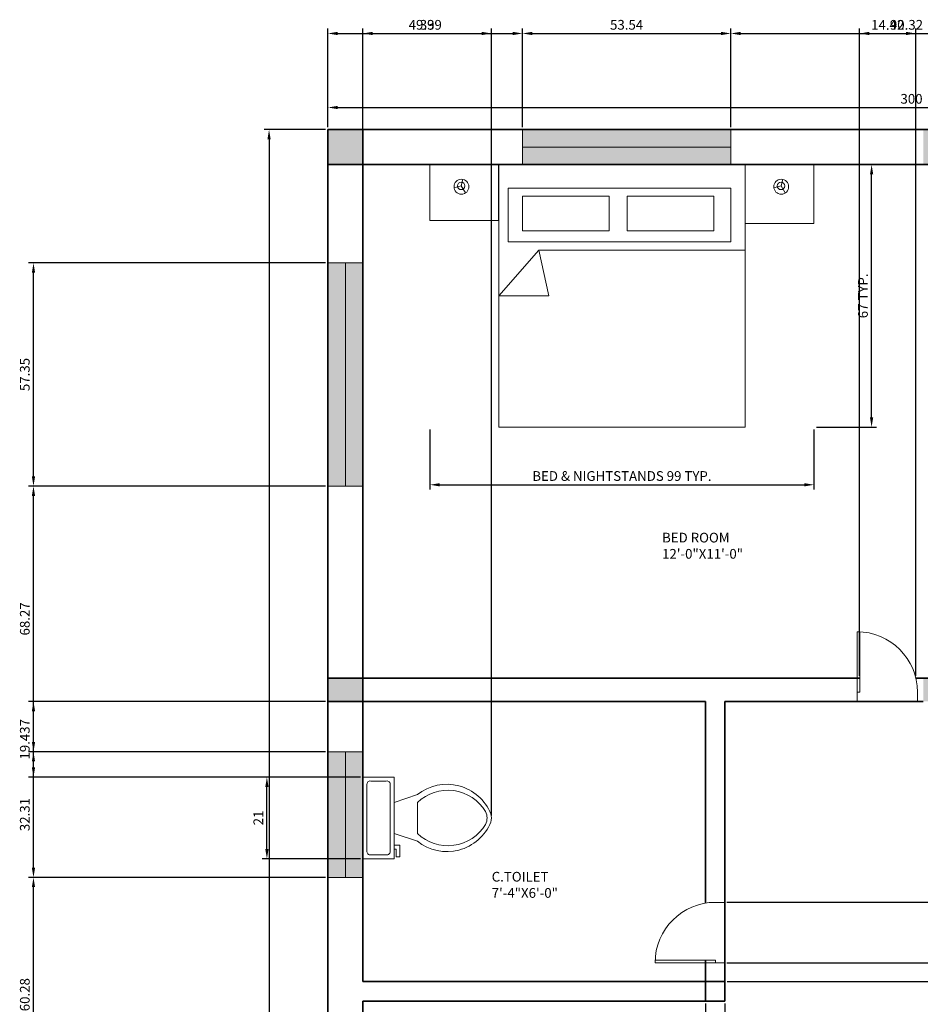
# Model space of a CAD drawing. Units: inches. Extents: x 33934 to 34340, y 20959 to 21493.
# Tile 3 of 4: x 33934 to 34166, y 21240 to 21493. Entities that reach past the tile are written whole.
import ezdxf

# ---------------------------------------------------------------- set-up
doc = ezdxf.new("R2010")
doc.units = ezdxf.units.IN
for name, color, linetype, lineweight in [('A-ANNO-DIMS', 2, 'Continuous', 18), ('A-AREA-IDEN', 7, 'Continuous', 18), ('A-DOOR', 3, 'Continuous', 18), ('A-FLOR-FIXT', 9, 'Continuous', 18), ('A-FURN', 8, 'Continuous', 18), ('A-GLAZ', 4, 'Continuous', 18), ('A-WALL', 7, 'Continuous', 35)]:
    doc.layers.add(name, color=color, linetype=linetype, lineweight=lineweight)
doc.layers.add('A-COLS-PATT', color=141, linetype='Continuous', lineweight=13, true_color=0xadddf7)
doc.layers.add('A-GLAZ-PATT', color=159, linetype='Continuous', lineweight=13, true_color=0x22346e)
doc.styles.get("Standard").update_dxf_attribs({"font": 'arial.ttf'})
doc.dimstyles.new('ISO-25', dxfattribs={"dimtxt": 2.5, "dimasz": 2.5, "dimexe": 1.25, "dimexo": 0.625, "dimtad": 1, "dimtxsty": 'Standard', "dimcen": 2.5, "dimadec": 0, "dimazin": 0, "dimtfac": 1, "dimtmove": 0, "dimatfit": 3, "dimfxl": 1, "dimarcsym": 0})

# ---------------------------------------------------------------- blocks, each defined once
blk = doc.blocks.new('*U3')
for p, q in [((9.5, -6), (9.5, -2)), ((-10, -8.5), (-8, -8.5)), ((-10, -9.5), (-10, -8.5)), ((-7, -9.5), (-10, -9.5)), ((-8, -8.5), (-8, -8)), ((-7, -8), (-7, -9.5)), ((-4, -8), (-6, -14)), ((4, -8), (6, -14)), ((4, -14), (-4, -14))]:
    blk.add_line(p, q)
blk.add_lwpolyline([(10.5, -8), (10.5, 0), (-10.5, 0), (-10.5, -8)], close=True)
for points in [[(-9.5, -2), (-9.5, -6)], [(8.5, -1), (-8.5, -1)], [(-8.5, -7), (8.5, -7)]]:
    blk.add_lwpolyline(points)
for centre, radius, start, end in [((-8.62, -1.88), 0.884, 81.8699, 188.1301), ((8.62, -1.88), 0.884, 351.8699, 98.1301), ((-8.62, -6.12), 0.884, 171.8699, 278.1301), ((8.62, -6.12), 0.884, 261.8699, 8.1301), ((3.52, -21.58), 12.17, 141.4691, 247.9714), ((4.2, -21.82), 11.33, 136.3677, 238.9468), ((-3.52, -21.58), 12.17, 292.0284, 38.5307), ((-4.2, -21.82), 11.33, 301.053, 43.6321), ((0, -27.88), 4, 245.7318, 294.2682), ((0, -29), 4, 254.8605, 285.1395)]:
    blk.add_arc(centre, radius, start, end)
blk = doc.blocks.new('*U5')
for p, q in [((0, 0), (0, -6)), ((40, 0), (40, -6))]:
    blk.add_line(p, q)
blk.add_lwpolyline([(0, 0), (0, 40), (1.75, 40), (1.75, 0)], close=True)
blk.add_arc((0, 0), 40, 0, 90)
blk = doc.blocks.new('*D6')
at = {"layer": 'A-ANNO-DIMS', "color": 0, "lineweight": -2, "transparency": 16777216}
for p, q in [((34013.69, 21465.74), (34013.69, 21472.03)), ((34313.69, 21465.74), (34313.69, 21472.03)), ((34016.19, 21470.78), (34311.19, 21470.78))]:
    blk.add_line(p, q, dxfattribs=at)
at = {"layer": 'A-ANNO-DIMS', "color": 0, "transparency": 16777216}
for points in [[(34016.19, 21471.2), (34016.19, 21470.37), (34013.69, 21470.78)], [(34311.19, 21471.2), (34311.19, 21470.37), (34313.69, 21470.78)]]:
    blk.add_solid(points, dxfattribs=at)
at = {"layer": 'Defpoints', "color": 0, "transparency": 16777216}
for p in [(34313.69, 21470.78), (34013.69, 21465.11), (34313.69, 21465.11)]:
    blk.add_point(p, dxfattribs=at)
at = {"layer": 'A-ANNO-DIMS', "color": 0, "transparency": 16777216, "insert": (34163.69, 21472.69), "char_height": 2.5, "attachment_point": 5}
blk.add_mtext('300', dxfattribs=at)
blk = doc.blocks.new('*D7')
at = {"layer": 'A-ANNO-DIMS', "color": 0, "lineweight": -2, "transparency": 16777216}
for p, q in [((34013.07, 21465.11), (33997.3, 21465.11)), ((33998.55, 21462.61), (33998.55, 20987.61)), ((34013.07, 20985.11), (33997.3, 20985.11))]:
    blk.add_line(p, q, dxfattribs=at)
at = {"layer": 'A-ANNO-DIMS', "color": 0, "transparency": 16777216}
for points in [[(33998.13, 21462.61), (33998.96, 21462.61), (33998.55, 21465.11)], [(33998.13, 20987.61), (33998.96, 20987.61), (33998.55, 20985.11)]]:
    blk.add_solid(points, dxfattribs=at)
at = {"layer": 'Defpoints', "color": 0, "transparency": 16777216}
for p in [(34013.69, 21465.11), (33998.55, 20985.11), (34013.69, 20985.11)]:
    blk.add_point(p, dxfattribs=at)
at = {"layer": 'A-ANNO-DIMS', "color": 0, "transparency": 16777216, "insert": (33996.64, 21225.11), "char_height": 2.5, "attachment_point": 5, "rotation": 90}
blk.add_mtext('480', dxfattribs=at)
blk = doc.blocks.new('BED-DOUBLE-WITH-NIGHTSTANDS')
for p, q in [((-9.63, -5.48), (-9.19, -3.82)), ((72.57, -5.48), (73, -3.82)), ((-9.63, -5.48), (-11.46, -5.95)), ((-9.63, -5.48), (-8.53, -7.28)), ((72.57, -5.48), (70.73, -5.95)), ((72.57, -5.48), (73.67, -7.28)), ((10.3, -21.96), (0, -33.74)), ((63.37, -21.96), (10.3, -21.96)), ((12.88, -33.74), (10.3, -21.96)), ((0, -33.74), (12.88, -33.74))]:
    blk.add_line(p, q)
for points in [[(-17.69, 0.01), (-0.01, 0.01), (-0.01, -14.39), (-17.69, -14.39)], [(0, 0), (63.37, 0), (63.37, -67.48), (0, -67.48)], [(63.36, 0.01), (81.04, 0.01), (81.04, -15.15), (63.36, -15.15)], [(2.46, -6.09), (59.71, -6.09), (59.71, -19.82), (2.46, -19.82)], [(6.09, -8.09), (28.36, -8.09), (28.36, -16.99), (6.09, -16.99)], [(33.05, -8.09), (55.31, -8.09), (55.31, -16.99), (33.05, -16.99)]]:
    blk.add_lwpolyline(points, close=True)
for centre, radius in [((-9.57, -5.69), 1.91), ((-9.63, -5.48), 0.951), ((72.62, -5.69), 1.91), ((72.57, -5.48), 0.951)]:
    blk.add_circle(centre, radius)
blk = doc.blocks.new('*D9')
at = {"layer": 'A-ANNO-DIMS', "color": 0, "lineweight": -2, "transparency": 16777216}
for p, q in [((34039.89, 21388), (34039.89, 21372.56)), ((34138.62, 21388), (34138.62, 21372.56)), ((34042.39, 21373.81), (34136.12, 21373.81))]:
    blk.add_line(p, q, dxfattribs=at)
at = {"layer": 'A-ANNO-DIMS', "color": 0, "transparency": 16777216}
for points in [[(34042.39, 21374.23), (34042.39, 21373.4), (34039.89, 21373.81)], [(34136.12, 21374.23), (34136.12, 21373.4), (34138.62, 21373.81)]]:
    blk.add_solid(points, dxfattribs=at)
at = {"layer": 'Defpoints', "color": 0, "transparency": 16777216}
for p in [(34039.89, 21388.62), (34138.62, 21388.62), (34138.62, 21373.81)]:
    blk.add_point(p, dxfattribs=at)
at = {"layer": 'A-ANNO-DIMS', "color": 0, "transparency": 16777216, "insert": (34089.25, 21375.74), "char_height": 2.5, "attachment_point": 5}
blk.add_mtext('BED & NIGHTSTANDS 99 TYP.', dxfattribs=at)
blk = doc.blocks.new('*D10')
at = {"layer": 'A-ANNO-DIMS', "color": 0, "lineweight": -2, "transparency": 16777216}
for p, q in [((34139.24, 21456.11), (34154.68, 21456.11)), ((34153.43, 21391.12), (34153.43, 21453.61)), ((34139.24, 21388.62), (34154.68, 21388.62))]:
    blk.add_line(p, q, dxfattribs=at)
at = {"layer": 'A-ANNO-DIMS', "color": 0, "transparency": 16777216}
for points in [[(34153.01, 21453.61), (34153.84, 21453.61), (34153.43, 21456.11)], [(34153.01, 21391.12), (34153.84, 21391.12), (34153.43, 21388.62)]]:
    blk.add_solid(points, dxfattribs=at)
at = {"layer": 'Defpoints', "color": 0, "transparency": 16777216}
for p in [(34138.62, 21456.11), (34153.43, 21456.11), (34138.62, 21388.62)]:
    blk.add_point(p, dxfattribs=at)
at = {"layer": 'A-ANNO-DIMS', "color": 0, "transparency": 16777216, "insert": (34151.53, 21422.37), "char_height": 2.5, "attachment_point": 5, "rotation": 90}
blk.add_mtext('67 TYP.', dxfattribs=at)
blk = doc.blocks.new('*D13')
at = {"layer": 'A-ANNO-DIMS', "color": 0, "lineweight": -2, "transparency": 16777216}
for p, q in [((34013.69, 21465.74), (34013.69, 21491.06)), ((34016.19, 21489.81), (34061.19, 21489.81)), ((34063.69, 21465.74), (34063.69, 21491.06))]:
    blk.add_line(p, q, dxfattribs=at)
at = {"layer": 'A-ANNO-DIMS', "color": 0, "transparency": 16777216}
for points in [[(34016.19, 21490.23), (34016.19, 21489.39), (34013.69, 21489.81)], [(34061.19, 21490.23), (34061.19, 21489.39), (34063.69, 21489.81)]]:
    blk.add_solid(points, dxfattribs=at)
at = {"layer": 'Defpoints', "color": 0, "transparency": 16777216}
for p in [(34063.69, 21489.81), (34013.69, 21465.11), (34063.69, 21465.11)]:
    blk.add_point(p, dxfattribs=at)
at = {"layer": 'A-ANNO-DIMS', "color": 0, "transparency": 16777216, "insert": (34038.69, 21491.71), "char_height": 2.5, "attachment_point": 5}
blk.add_mtext('49.99', dxfattribs=at)
blk = doc.blocks.new('*D14')
at = {"layer": 'A-ANNO-DIMS', "color": 0, "lineweight": -2, "transparency": 16777216}
for p, q in [((34063.69, 21465.74), (34063.69, 21491.06)), ((34066.19, 21489.81), (34114.73, 21489.81)), ((34117.23, 21465.74), (34117.23, 21491.06))]:
    blk.add_line(p, q, dxfattribs=at)
at = {"layer": 'A-ANNO-DIMS', "color": 0, "transparency": 16777216}
for points in [[(34066.19, 21490.23), (34066.19, 21489.39), (34063.69, 21489.81)], [(34114.73, 21490.23), (34114.73, 21489.39), (34117.23, 21489.81)]]:
    blk.add_solid(points, dxfattribs=at)
at = {"layer": 'Defpoints', "color": 0, "transparency": 16777216}
for p in [(34117.23, 21489.81), (34063.69, 21465.11), (34117.23, 21465.11)]:
    blk.add_point(p, dxfattribs=at)
at = {"layer": 'A-ANNO-DIMS', "color": 0, "transparency": 16777216, "insert": (34090.46, 21491.71), "char_height": 2.5, "attachment_point": 5}
blk.add_mtext('53.54', dxfattribs=at)
blk = doc.blocks.new('*D15')
at = {"layer": 'A-ANNO-DIMS', "color": 0, "lineweight": -2, "transparency": 16777216}
for p, q in [((34117.23, 21465.74), (34117.23, 21491.06)), ((34119.73, 21489.81), (34205.05, 21489.81)), ((34207.55, 21465.74), (34207.55, 21491.06))]:
    blk.add_line(p, q, dxfattribs=at)
at = {"layer": 'A-ANNO-DIMS', "color": 0, "transparency": 16777216}
for points in [[(34119.73, 21490.23), (34119.73, 21489.39), (34117.23, 21489.81)], [(34205.05, 21490.23), (34205.05, 21489.39), (34207.55, 21489.81)]]:
    blk.add_solid(points, dxfattribs=at)
at = {"layer": 'Defpoints', "color": 0, "transparency": 16777216}
for p in [(34207.55, 21489.81), (34117.23, 21465.11), (34207.55, 21465.11)]:
    blk.add_point(p, dxfattribs=at)
at = {"layer": 'A-ANNO-DIMS', "color": 0, "transparency": 16777216, "insert": (34162.39, 21491.71), "char_height": 2.5, "attachment_point": 5}
blk.add_mtext('90.32', dxfattribs=at)
blk = doc.blocks.new('*D19')
at = {"layer": 'A-ANNO-DIMS', "color": 0, "lineweight": -2, "transparency": 16777216}
for p, q in [((34013.07, 21272.89), (33936.74, 21272.89)), ((33937.99, 21215.11), (33937.99, 21270.39)), ((34013.07, 21212.61), (33936.74, 21212.61))]:
    blk.add_line(p, q, dxfattribs=at)
at = {"layer": 'A-ANNO-DIMS', "color": 0, "transparency": 16777216}
for points in [[(33937.58, 21270.39), (33938.41, 21270.39), (33937.99, 21272.89)], [(33937.58, 21215.11), (33938.41, 21215.11), (33937.99, 21212.61)]]:
    blk.add_solid(points, dxfattribs=at)
at = {"layer": 'Defpoints', "color": 0, "transparency": 16777216}
for p in [(33937.99, 21272.89), (34013.69, 21272.89), (34013.69, 21212.61)]:
    blk.add_point(p, dxfattribs=at)
at = {"layer": 'A-ANNO-DIMS', "color": 0, "transparency": 16777216, "insert": (33936.09, 21242.75), "char_height": 2.5, "attachment_point": 5, "rotation": 90}
blk.add_mtext('60.28', dxfattribs=at)
blk = doc.blocks.new('*D20')
at = {"layer": 'A-ANNO-DIMS', "color": 0, "lineweight": -2, "transparency": 16777216}
for p, q in [((34013.07, 21305.2), (33936.74, 21305.2)), ((33937.99, 21275.39), (33937.99, 21302.7)), ((34013.07, 21272.89), (33936.74, 21272.89))]:
    blk.add_line(p, q, dxfattribs=at)
at = {"layer": 'A-ANNO-DIMS', "color": 0, "transparency": 16777216}
for points in [[(33937.58, 21302.7), (33938.41, 21302.7), (33937.99, 21305.2)], [(33937.58, 21275.39), (33938.41, 21275.39), (33937.99, 21272.89)]]:
    blk.add_solid(points, dxfattribs=at)
at = {"layer": 'Defpoints', "color": 0, "transparency": 16777216}
for p in [(33937.99, 21305.2), (34013.69, 21305.2), (34013.69, 21272.89)]:
    blk.add_point(p, dxfattribs=at)
at = {"layer": 'A-ANNO-DIMS', "color": 0, "transparency": 16777216, "insert": (33936.09, 21289.05), "char_height": 2.5, "attachment_point": 5, "rotation": 90}
blk.add_mtext('32.31', dxfattribs=at)
blk = doc.blocks.new('*D21')
at = {"layer": 'A-ANNO-DIMS', "color": 0, "lineweight": -2, "transparency": 16777216}
for p, q in [((34013.07, 21373.47), (33936.74, 21373.47)), ((33937.99, 21307.7), (33937.99, 21370.97)), ((34013.07, 21305.2), (33936.74, 21305.2))]:
    blk.add_line(p, q, dxfattribs=at)
at = {"layer": 'A-ANNO-DIMS', "color": 0, "transparency": 16777216}
for points in [[(33937.58, 21370.97), (33938.41, 21370.97), (33937.99, 21373.47)], [(33937.58, 21307.7), (33938.41, 21307.7), (33937.99, 21305.2)]]:
    blk.add_solid(points, dxfattribs=at)
at = {"layer": 'Defpoints', "color": 0, "transparency": 16777216}
for p in [(33937.99, 21373.47), (34013.69, 21373.47), (34013.69, 21305.2)]:
    blk.add_point(p, dxfattribs=at)
at = {"layer": 'A-ANNO-DIMS', "color": 0, "transparency": 16777216, "insert": (33936.09, 21339.34), "char_height": 2.5, "attachment_point": 5, "rotation": 90}
blk.add_mtext('68.27', dxfattribs=at)
blk = doc.blocks.new('*D22')
at = {"layer": 'A-ANNO-DIMS', "color": 0, "lineweight": -2, "transparency": 16777216}
for p, q in [((34013.07, 21430.82), (33936.74, 21430.82)), ((33937.99, 21375.97), (33937.99, 21428.32)), ((34013.07, 21373.47), (33936.74, 21373.47))]:
    blk.add_line(p, q, dxfattribs=at)
at = {"layer": 'A-ANNO-DIMS', "color": 0, "transparency": 16777216}
for points in [[(33937.58, 21428.32), (33938.41, 21428.32), (33937.99, 21430.82)], [(33937.58, 21375.97), (33938.41, 21375.97), (33937.99, 21373.47)]]:
    blk.add_solid(points, dxfattribs=at)
at = {"layer": 'Defpoints', "color": 0, "transparency": 16777216}
for p in [(33937.99, 21430.82), (34013.69, 21430.82), (34013.69, 21373.47)]:
    blk.add_point(p, dxfattribs=at)
at = {"layer": 'A-ANNO-DIMS', "color": 0, "transparency": 16777216, "insert": (33936.09, 21402.15), "char_height": 2.5, "attachment_point": 5, "rotation": 90}
blk.add_mtext('57.35', dxfattribs=at)
blk = doc.blocks.new('*D41')
at = {"layer": 'A-ANNO-DIMS', "color": 0, "lineweight": -2, "transparency": 16777216}
for p, q in [((34150.36, 21324.74), (34150.36, 21491.06)), ((34152.86, 21489.81), (34162.28, 21489.81)), ((34164.78, 21324.74), (34164.78, 21491.06))]:
    blk.add_line(p, q, dxfattribs=at)
at = {"layer": 'A-ANNO-DIMS', "color": 0, "transparency": 16777216}
for points in [[(34152.86, 21490.23), (34152.86, 21489.39), (34150.36, 21489.81)], [(34162.28, 21490.23), (34162.28, 21489.39), (34164.78, 21489.81)]]:
    blk.add_solid(points, dxfattribs=at)
at = {"layer": 'Defpoints', "color": 0, "transparency": 16777216}
for p in [(34164.78, 21489.81), (34150.36, 21324.11), (34164.78, 21324.11)]:
    blk.add_point(p, dxfattribs=at)
at = {"layer": 'A-ANNO-DIMS', "color": 0, "transparency": 16777216, "insert": (34157.57, 21491.69), "char_height": 2.5, "attachment_point": 5}
blk.add_mtext('14.42', dxfattribs=at)
blk = doc.blocks.new('*D43')
at = {"layer": 'A-ANNO-DIMS', "color": 0, "lineweight": -2, "transparency": 16777216}
for p, q in [((34022.69, 21299.3), (34022.69, 21491.06)), ((34025.19, 21489.81), (34053.19, 21489.81)), ((34055.69, 21288.8), (34055.69, 21491.06))]:
    blk.add_line(p, q, dxfattribs=at)
at = {"layer": 'A-ANNO-DIMS', "color": 0, "transparency": 16777216}
for points in [[(34025.19, 21490.23), (34025.19, 21489.39), (34022.69, 21489.81)], [(34053.19, 21490.23), (34053.19, 21489.39), (34055.69, 21489.81)]]:
    blk.add_solid(points, dxfattribs=at)
at = {"layer": 'Defpoints', "color": 0, "transparency": 16777216}
for p in [(34055.69, 21489.81), (34022.69, 21298.67), (34055.69, 21288.17)]:
    blk.add_point(p, dxfattribs=at)
at = {"layer": 'A-ANNO-DIMS', "color": 0, "transparency": 16777216, "insert": (34039.19, 21491.71), "char_height": 2.5, "attachment_point": 5}
blk.add_mtext('33', dxfattribs=at)
blk = doc.blocks.new('*D44')
at = {"layer": 'A-ANNO-DIMS', "color": 0, "lineweight": -2, "transparency": 16777216}
for p, q in [((34022.07, 21298.67), (33996.74, 21298.67)), ((33997.99, 21280.17), (33997.99, 21296.17)), ((34022.07, 21277.67), (33996.74, 21277.67))]:
    blk.add_line(p, q, dxfattribs=at)
at = {"layer": 'A-ANNO-DIMS', "color": 0, "transparency": 16777216}
for points in [[(33997.58, 21296.17), (33998.41, 21296.17), (33997.99, 21298.67)], [(33997.58, 21280.17), (33998.41, 21280.17), (33997.99, 21277.67)]]:
    blk.add_solid(points, dxfattribs=at)
at = {"layer": 'Defpoints', "color": 0, "transparency": 16777216}
for p in [(33997.99, 21298.67), (34022.69, 21298.67), (34022.69, 21277.67)]:
    blk.add_point(p, dxfattribs=at)
at = {"layer": 'A-ANNO-DIMS', "color": 0, "transparency": 16777216, "insert": (33996.11, 21288.17), "char_height": 2.5, "attachment_point": 5, "rotation": 90}
blk.add_mtext('21', dxfattribs=at)
blk = doc.blocks.new('*D45')
at = {"layer": 'A-ANNO-DIMS', "color": 0, "lineweight": -2, "transparency": 16777216}
for p, q in [((34013.07, 21318.11), (33936.74, 21318.11)), ((33937.99, 21301.17), (33937.99, 21315.61)), ((34022.07, 21298.67), (33936.74, 21298.67))]:
    blk.add_line(p, q, dxfattribs=at)
at = {"layer": 'A-ANNO-DIMS', "color": 0, "transparency": 16777216}
for points in [[(33937.58, 21315.61), (33938.41, 21315.61), (33937.99, 21318.11)], [(33937.58, 21301.17), (33938.41, 21301.17), (33937.99, 21298.67)]]:
    blk.add_solid(points, dxfattribs=at)
at = {"layer": 'Defpoints', "color": 0, "transparency": 16777216}
for p in [(33937.99, 21318.11), (34013.69, 21318.11), (34022.69, 21298.67)]:
    blk.add_point(p, dxfattribs=at)
at = {"layer": 'A-ANNO-DIMS', "color": 0, "transparency": 16777216, "insert": (33936.09, 21308.39), "char_height": 2.5, "attachment_point": 5, "rotation": 90}
blk.add_mtext('19.437', dxfattribs=at)
blk = doc.blocks.new('*D46')
at = {"layer": 'A-ANNO-DIMS', "color": 0, "lineweight": -2, "transparency": 16777216}
for p, q in [((34116.25, 21266.49), (34339.64, 21266.49)), ((34338.39, 21253.47), (34338.39, 21263.99)), ((34116.25, 21250.97), (34339.64, 21250.97))]:
    blk.add_line(p, q, dxfattribs=at)
at = {"layer": 'A-ANNO-DIMS', "color": 0, "transparency": 16777216}
for points in [[(34337.98, 21263.99), (34338.81, 21263.99), (34338.39, 21266.49)], [(34337.98, 21253.47), (34338.81, 21253.47), (34338.39, 21250.97)]]:
    blk.add_solid(points, dxfattribs=at)
at = {"layer": 'Defpoints', "color": 0, "transparency": 16777216}
for p in [(34115.62, 21266.49), (34338.39, 21266.49), (34115.62, 21250.97)]:
    blk.add_point(p, dxfattribs=at)
at = {"layer": 'A-ANNO-DIMS', "color": 0, "transparency": 16777216, "insert": (34336.49, 21258.73), "char_height": 2.5, "attachment_point": 5, "rotation": 90}
blk.add_mtext('15.52', dxfattribs=at)
blk = doc.blocks.new('*D47')
at = {"layer": 'A-ANNO-DIMS', "color": 0, "lineweight": -2, "transparency": 16777216}
for p, q in [((34338.39, 21253.47), (34338.39, 21265.75)), ((34116.25, 21250.97), (34339.64, 21250.97)), ((34338.39, 21246.11), (34338.39, 21250.97)), ((34116.32, 21246.11), (34339.64, 21246.11)), ((34338.39, 21243.61), (34338.39, 21241.11))]:
    blk.add_line(p, q, dxfattribs=at)
at = {"layer": 'A-ANNO-DIMS', "color": 0, "transparency": 16777216}
for points in [[(34337.98, 21253.47), (34338.81, 21253.47), (34338.39, 21250.97)], [(34337.98, 21243.61), (34338.81, 21243.61), (34338.39, 21246.11)]]:
    blk.add_solid(points, dxfattribs=at)
at = {"layer": 'Defpoints', "color": 0, "transparency": 16777216}
for p in [(34115.62, 21250.97), (34338.39, 21250.97), (34115.69, 21246.11)]:
    blk.add_point(p, dxfattribs=at)
at = {"layer": 'A-ANNO-DIMS', "color": 0, "transparency": 16777216, "insert": (34336.49, 21260.86), "char_height": 2.5, "attachment_point": 5, "rotation": 90}
blk.add_mtext('4.856', dxfattribs=at)
blk = doc.blocks.new('*D51')
at = {"layer": 'A-ANNO-DIMS', "color": 0, "lineweight": -2, "transparency": 16777216}
for p, q in [((34110.69, 21240.49), (34110.69, 20959.15)), ((34115.69, 21240.49), (34115.69, 20959.15)), ((34108.19, 20960.4), (34105.69, 20960.4)), ((34110.69, 20960.4), (34115.69, 20960.4)), ((34118.19, 20960.4), (34120.69, 20960.4))]:
    blk.add_line(p, q, dxfattribs=at)
at = {"layer": 'A-ANNO-DIMS', "color": 0, "transparency": 16777216}
for points in [[(34108.19, 20960.81), (34108.19, 20959.98), (34110.69, 20960.4)], [(34118.19, 20960.81), (34118.19, 20959.98), (34115.69, 20960.4)]]:
    blk.add_solid(points, dxfattribs=at)
at = {"layer": 'Defpoints', "color": 0, "transparency": 16777216}
for p in [(34110.69, 21241.11), (34115.69, 21241.11), (34115.69, 20960.4)]:
    blk.add_point(p, dxfattribs=at)
at = {"layer": 'A-ANNO-DIMS', "color": 0, "transparency": 16777216, "insert": (34113.19, 20962.29), "char_height": 2.5, "attachment_point": 5}
blk.add_mtext('5', dxfattribs=at)

msp = doc.modelspace()

# ---------------------------------------------------------------- hatches: boundary and pattern name
at = {"layer": 'A-COLS-PATT'}
h = msp.add_hatch(color=256, dxfattribs=at)
h.dxf.hatch_style = 1
h.paths.add_polyline_path([(34022.6921, 20994.1104), (34013.6921, 20994.1104), (34013.6921, 20985.1104), (34022.6921, 20985.1104)])
h.paths.add_polyline_path([(34163.6921, 20994.1104), (34158.6922, 20994.1104), (34158.6922, 20985.1104), (34163.6921, 20985.1104)])
h.paths.add_polyline_path([(34313.6921, 20994.1104), (34304.6921, 20994.1104), (34304.6921, 20985.1104), (34313.6921, 20985.1104)])
h.paths.add_polyline_path([(34313.6921, 21077.1104), (34304.6921, 21077.1104), (34304.6921, 21072.1104), (34313.6921, 21072.1104)])
h.paths.add_polyline_path([(34172.6921, 21077.1104), (34167.6921, 21077.1104), (34167.6921, 21072.1104), (34172.6921, 21072.1104)])
h.paths.add_polyline_path([(34022.6921, 21324.1104), (34013.6921, 21324.1104), (34013.6921, 21318.1104), (34022.6921, 21318.1104)])
h.paths.add_polyline_path([(34171.6921, 21324.1104), (34166.6921, 21324.1104), (34166.6921, 21318.1104), (34171.6921, 21318.1104)])
h.paths.add_polyline_path([(34313.6921, 21282.1104), (34304.6921, 21282.1104), (34304.6921, 21277.1104), (34313.6921, 21277.1104)])
h.paths.add_polyline_path([(34313.6921, 21465.1104), (34304.6921, 21465.1104), (34304.6921, 21456.1104), (34313.6921, 21456.1104)])
h.paths.add_polyline_path([(34171.6921, 21465.1104), (34166.6921, 21465.1104), (34166.6921, 21456.1104), (34171.6921, 21456.1104)])
h.paths.add_polyline_path([(34022.6921, 21465.1104), (34013.6921, 21465.1104), (34013.6921, 21456.1104), (34022.6921, 21456.1104)])
at = {"layer": 'A-GLAZ-PATT'}
h = msp.add_hatch(color=256, dxfattribs=at)
h.dxf.hatch_style = 1
h.paths.add_polyline_path([(34022.6921, 21212.6089), (34018.1921, 21212.6089), (34018.1921, 21149.8921), (34022.6921, 21149.8921)])
h.paths.add_polyline_path([(34018.1921, 21212.6089), (34013.6921, 21212.6089), (34013.6921, 21149.8921), (34018.1921, 21149.8921)])
h.paths.add_polyline_path([(34142.0454, 21077.1104), (34099.5314, 21077.1104), (34099.5314, 21074.6104), (34142.0454, 21074.6104)])
h.paths.add_polyline_path([(34142.0454, 21074.6104), (34099.5314, 21074.6104), (34099.5314, 21072.1104), (34142.0454, 21072.1104)])
h.paths.add_polyline_path([(34313.6921, 21160.1148), (34309.1921, 21160.1148), (34309.1921, 21107.9155), (34313.6921, 21107.9155)])
h.paths.add_polyline_path([(34309.1921, 21160.1148), (34304.6921, 21160.1148), (34304.6921, 21107.9155), (34309.1921, 21107.9155)])
h.paths.add_polyline_path([(34309.1921, 21244.1846), (34304.6921, 21244.1846), (34304.6921, 21212.6883), (34309.1921, 21212.6883)])
h.paths.add_polyline_path([(34313.6921, 21244.1846), (34309.1921, 21244.1846), (34309.1921, 21212.6883), (34313.6921, 21212.6883)])
h.paths.add_polyline_path([(34313.6921, 21394.9809), (34309.1921, 21394.9809), (34309.1921, 21355.1902), (34313.6921, 21355.1902)])
h.paths.add_polyline_path([(34309.1921, 21394.9809), (34304.6921, 21394.9809), (34304.6921, 21355.1902), (34309.1921, 21355.1902)])
h.paths.add_polyline_path([(34257.3396, 21465.1104), (34207.5515, 21465.1104), (34207.5515, 21460.6104), (34257.3396, 21460.6104)])
h.paths.add_polyline_path([(34257.3396, 21460.6104), (34207.5515, 21460.6104), (34207.5515, 21456.1104), (34257.3396, 21456.1104)])
h.paths.add_polyline_path([(34117.2268, 21465.1104), (34063.6855, 21465.1104), (34063.6855, 21460.6104), (34117.2268, 21460.6104)])
h.paths.add_polyline_path([(34117.2268, 21460.6104), (34063.6855, 21460.6104), (34063.6855, 21456.1104), (34117.2268, 21456.1104)])
h.paths.add_polyline_path([(34022.6921, 21430.8215), (34018.1921, 21430.8215), (34018.1921, 21373.469), (34022.6921, 21373.469)])
h.paths.add_polyline_path([(34018.1921, 21430.8215), (34013.6921, 21430.8215), (34013.6921, 21373.469), (34018.1921, 21373.469)])
h.paths.add_polyline_path([(34018.1921, 21305.2021), (34013.6921, 21305.2021), (34013.6921, 21272.8905), (34018.1921, 21272.8905)])
h.paths.add_polyline_path([(34022.6921, 21305.2021), (34018.1921, 21305.2021), (34018.1921, 21272.8905), (34022.6921, 21272.8905)])

# ---------------------------------------------------------------- linework, layer by layer
at = {"layer": 'A-GLAZ'}
for p, q in [((34063.6855, 21465.1104), (34063.6855, 21456.1104)), ((34117.2268, 21456.1104), (34117.2268, 21465.1104)), ((34117.2268, 21465.1104), (34117.2268, 21460.6104)), ((34117.2268, 21460.6104), (34063.6855, 21460.6104)), ((34063.6855, 21456.1104), (34117.2268, 21456.1104)), ((34022.6921, 21430.8215), (34013.6921, 21430.8215)), ((34013.6921, 21430.8215), (34013.6921, 21373.469)), ((34018.1921, 21373.469), (34018.1921, 21430.8215)), ((34013.6921, 21373.469), (34022.6921, 21373.469)), ((34022.6921, 21373.469), (34018.1921, 21373.469)), ((34022.6921, 21305.2021), (34013.6921, 21305.2021)), ((34013.6921, 21305.2021), (34013.6921, 21272.8905)), ((34018.1921, 21272.8905), (34018.1921, 21305.2021)), ((34013.6921, 21272.8905), (34022.6921, 21272.8905)), ((34022.6921, 21272.8905), (34018.1921, 21272.8905))]:
    msp.add_line(p, q, dxfattribs=at)
at = {"layer": 'A-WALL'}
for p, q in [((34013.6921, 21465.1104), (34313.6921, 21465.1104)), ((34013.6921, 20985.1104), (34013.6921, 21465.1104)), ((34022.6921, 21246.1104), (34022.6921, 21465.1104)), ((34013.6921, 21456.1104), (34313.6921, 21456.1104)), ((34013.6921, 21324.1104), (34150.3627, 21324.1104)), ((34164.7827, 21324.1104), (34171.6921, 21324.1104)), ((34013.6921, 21318.1104), (34110.6921, 21318.1104)), ((34110.6921, 21266.2672), (34110.6921, 21318.1104)), ((34115.6921, 21241.1104), (34115.6921, 21318.1104)), ((34115.6921, 21318.1104), (34166.6921, 21318.1104)), ((34110.6921, 21241.1104), (34110.6921, 21251.6458)), ((34022.6921, 21246.1104), (34115.6921, 21246.1104)), ((34022.6921, 20985.1104), (34022.6921, 21241.1104)), ((34022.6921, 21241.1104), (34115.6921, 21241.1104))]:
    msp.add_line(p, q, dxfattribs=at)

# ---------------------------------------------------------------- block references
at = {"layer": 'A-DOOR', "xscale": 0.3880097502641484, "yscale": 0.3880097502641484, "zscale": 0.3880097502641484}
msp.add_blockref('*U5', (34149.6837, 21320.5183), dxfattribs=at)
at = {"layer": 'A-DOOR', "xscale": 0.3880097502641484, "yscale": 0.3880097502641484, "zscale": 0.3880097502641484, "rotation": 90}
msp.add_blockref('*U5', (34113.2957, 21250.9668), dxfattribs=at)
at = {"layer": 'A-FLOR-FIXT', "rotation": 89.99999999999999}
msp.add_blockref('*U3', (34022.6921, 21288.1736), dxfattribs=at)
at = {"layer": 'A-FURN'}
msp.add_blockref('BED-DOUBLE-WITH-NIGHTSTANDS', (34057.5742, 21456.1023), dxfattribs=at)

# ---------------------------------------------------------------- texts
at = {"layer": 'A-AREA-IDEN', "char_height": 2.5, "attachment_point": 1}
for s, width, insert in [('BED ROOM\\P12\'-0"X11\'-0"', 46.425798, (34099.5702, 21361.48)), ('C.TOILET\\P7\'-4"X6\'-0"', 33.487249, (34055.7759, 21274.3218))]:
    msp.add_mtext_dynamic_manual_height_columns(s, width=width, gutter_width=12.5, heights=[0], dxfattribs=dict(at, insert=insert))

# ---------------------------------------------------------------- dimensions: what is measured, and where the dimension line sits
at = {"layer": 'A-ANNO-DIMS'}
for base, p1, p2, override, picture, middle in [((34063.6855, 21489.8104), (34013.6921, 21465.1104), (34063.6855, 21465.1104), {"dimdec": 2, "dimlfac": 1, "dimrnd": 0, "dimzin": 0, "dimdsep": 46, "dimlunit": 2}, '*D13', (34038.6888, 21491.7119)), ((34055.6921, 21489.8104), (34022.6921, 21298.6736), (34055.6921, 21288.1736), {"dimdec": 0, "dimlfac": 1, "dimrnd": 0, "dimzin": 0, "dimdsep": 46, "dimlunit": 2}, '*D43', (34039.1921, 21491.7127)), ((34117.2268, 21489.8104), (34063.6855, 21465.1104), (34117.2268, 21465.1104), {"dimdec": 2, "dimlfac": 1, "dimrnd": 0, "dimzin": 0, "dimdsep": 46, "dimlunit": 2}, '*D14', (34090.4562, 21491.7127)), ((34207.5515, 21489.8104), (34117.2268, 21465.1104), (34207.5515, 21465.1104), {"dimdec": 2, "dimlfac": 1, "dimrnd": 0, "dimzin": 0, "dimdsep": 46, "dimlunit": 2}, '*D15', (34162.3892, 21491.7127)), ((34164.7827, 21489.8104), (34150.3627, 21324.1104), (34164.7827, 21324.1104), {"dimdec": 2, "dimlfac": 1, "dimrnd": 0, "dimzin": 0, "dimdsep": 46, "dimlunit": 2}, '*D41', (34157.5727, 21491.6906)), ((34313.6921, 21470.7844), (34013.6921, 21465.1104), (34313.6921, 21465.1104), {"dimclrd": 0, "dimclre": 0, "dimclrt": 0}, '*D6', (34163.6921, 21472.6867)), ((34115.6921, 20960.3981), (34110.6921, 21241.1104), (34115.6921, 21241.1104), {"dimdec": 0, "dimlfac": 1, "dimrnd": 0, "dimzin": 0, "dimdsep": 46, "dimlunit": 2}, '*D51', (34113.1921, 20962.2944))]:
    dim = msp.add_linear_dim(base=base, p1=p1, p2=p2, dimstyle='ISO-25', override=override, dxfattribs=at)
    dim.commit()
    dim.dimension.update_dxf_attribs({"geometry": picture, "text_midpoint": middle})
for base, p1, p2, override, picture, middle in [((33998.546, 20985.1104), (34013.6921, 21465.1104), (34013.6921, 20985.1104), {"dimclrd": 0, "dimclre": 0, "dimclrt": 0}, '*D7', (33996.6445, 21225.1104)), ((33937.9921, 21430.8215), (34013.6921, 21373.469), (34013.6921, 21430.8215), {"dimdec": 2, "dimlfac": 1, "dimrnd": 0, "dimzin": 0, "dimdsep": 46, "dimlunit": 2}, '*D22', (33936.0899, 21402.1452)), ((33937.9921, 21373.469), (34013.6921, 21305.2021), (34013.6921, 21373.469), {"dimdec": 2, "dimlfac": 1, "dimrnd": 0, "dimzin": 0, "dimdsep": 46, "dimlunit": 2}, '*D21', (33936.0907, 21339.3356)), ((33937.9921, 21318.1104), (34022.6921, 21298.6736), (34013.6921, 21318.1104), {"dimdec": 3, "dimlfac": 1, "dimrnd": 0, "dimzin": 0, "dimdsep": 46, "dimlunit": 2}, '*D45', (33936.0899, 21308.392)), ((33937.9921, 21305.2021), (34013.6921, 21272.8905), (34013.6921, 21305.2021), {"dimdec": 2, "dimlfac": 1, "dimrnd": 0, "dimzin": 0, "dimdsep": 46, "dimlunit": 2}, '*D20', (33936.0899, 21289.0463)), ((33997.9921, 21298.6736), (34022.6921, 21277.6736), (34022.6921, 21298.6736), {"dimdec": 0, "dimlfac": 1, "dimrnd": 0, "dimzin": 0, "dimdsep": 46, "dimlunit": 2}, '*D44', (33996.112, 21288.1736)), ((33937.9921, 21272.8905), (34013.6921, 21212.6089), (34013.6921, 21272.8905), {"dimdec": 2, "dimlfac": 1, "dimrnd": 0, "dimzin": 0, "dimdsep": 46, "dimlunit": 2}, '*D19', (33936.0907, 21242.7497)), ((34338.3921, 21266.4872), (34115.6238, 21250.9668), (34115.6238, 21266.4872), {"dimdec": 2, "dimlfac": 1, "dimrnd": 0, "dimzin": 0, "dimdsep": 46, "dimlunit": 2}, '*D46', (34336.4907, 21258.727)), ((34338.3921, 21250.9668), (34115.6921, 21246.1104), (34115.6238, 21250.9668), {"dimdec": 3, "dimlfac": 1, "dimrnd": 0, "dimzin": 0, "dimdsep": 46, "dimlunit": 2}, '*D47', (34336.4907, 21260.8593))]:
    dim = msp.add_linear_dim(base=base, p1=p1, p2=p2, angle=90, dimstyle='ISO-25', override=override, dxfattribs=at)
    dim.commit()
    dim.dimension.update_dxf_attribs({"geometry": picture, "text_midpoint": middle})
dim = msp.add_linear_dim(base=(34153.4283, 21456.1104), p1=(34138.6184, 21388.6215), p2=(34138.6184, 21456.1104), angle=90, text='<> TYP.', dimstyle='ISO-25', override={"dimdec": 0, "dimlfac": 1, "dimrnd": 0, "dimzin": 0, "dimdsep": 46, "dimlunit": 2}, dxfattribs=at)
dim.commit()
dim.dimension.update_dxf_attribs({"geometry": '*D10', "text_midpoint": (34151.5268, 21422.366)})
dim = msp.add_linear_dim(base=(34138.6184, 21373.8117), p1=(34039.8862, 21388.6215), p2=(34138.6184, 21388.6215), text='BED & NIGHTSTANDS <> TYP.', dimstyle='ISO-25', override={"dimdec": 0, "dimlfac": 1, "dimrnd": 0, "dimzin": 0, "dimdsep": 46, "dimlunit": 2}, dxfattribs=at)
dim.commit()
dim.dimension.update_dxf_attribs({"geometry": '*D9', "text_midpoint": (34089.2523, 21375.737)})

doc.saveas('drawing.dxf')
